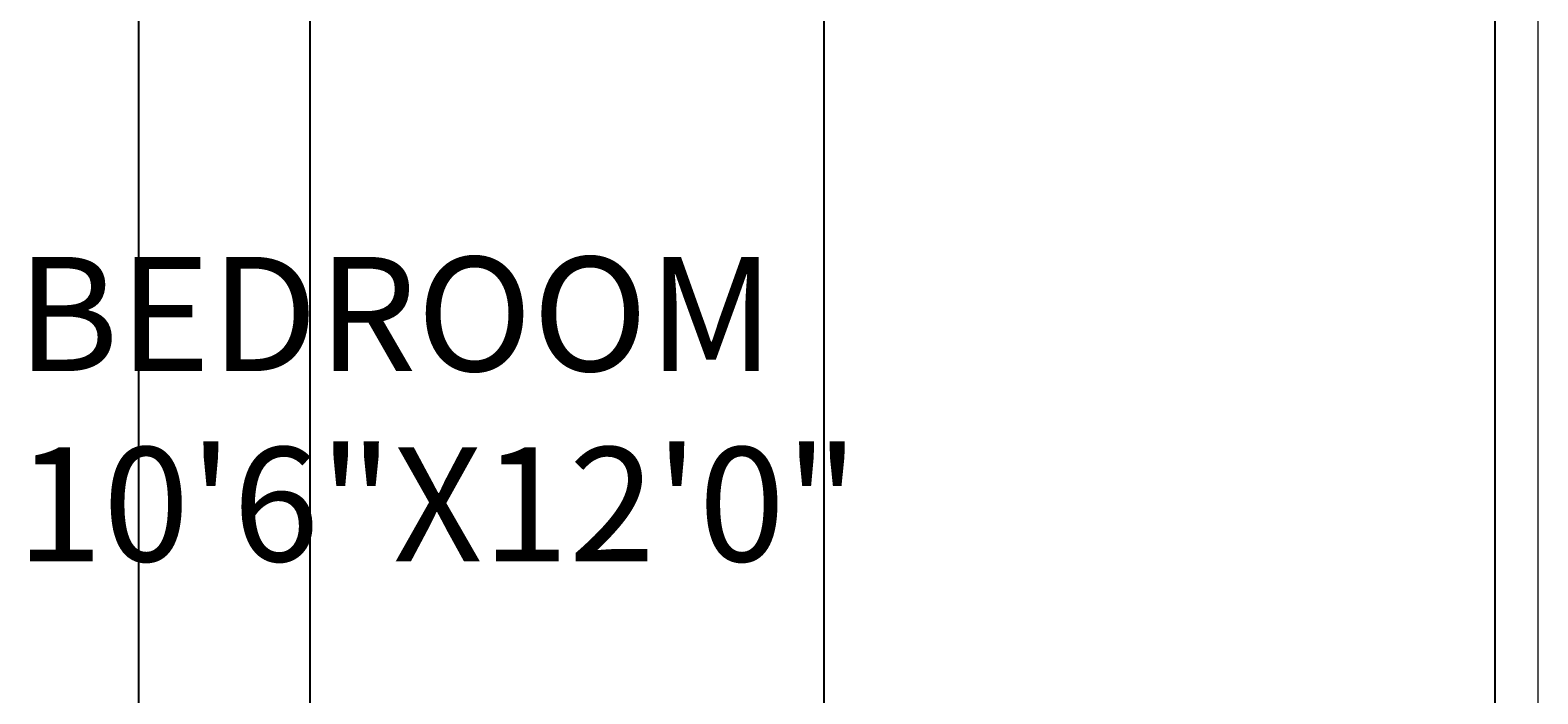
# Model space of a CAD drawing. Units: inches. Extents: x 1088 to 1703, y 668 to 1875.
# Tile 28 of 45: x 1509 to 1588, y 1504 to 1539. Entities that reach past the tile are written whole.
import ezdxf

# ---------------------------------------------------------------- set-up
doc = ezdxf.new("R2010")
doc.units = ezdxf.units.IN
for name, color, linetype, lineweight in [('A-ANNO-DIMS', 2, 'Continuous', 18), ('A-AREA-IDEN', 7, 'Continuous', 18), ('A-DOOR', 4, 'Continuous', 18)]:
    doc.layers.add(name, color=color, linetype=linetype, lineweight=lineweight)
doc.styles.get("Standard").update_dxf_attribs({"font": 'arial.ttf'})
doc.dimstyles.get("Standard").update_dxf_attribs({"dimtxt": 0.18, "dimasz": 0.18, "dimexe": 0.18, "dimexo": 0.0625, "dimgap": 0.09, "dimtad": 0, "dimtih": 1, "dimtoh": 1, "dimdec": 4, "dimzin": 0, "dimdsep": 46, "dimtxsty": 'Standard', "dimcen": 0.09, "dimadec": 0, "dimazin": 0, "dimtfac": 1, "dimtdec": 4, "dimtofl": 0, "dimtmove": 0, "dimatfit": 3, "dimfxl": 1, "dimtolj": 1, "dimtzin": 0, "dimarcsym": 0})

# ---------------------------------------------------------------- blocks, each defined once
blk = doc.blocks.new('*D32')
at = {"layer": 'A-ANNO-DIMS', "color": 0, "lineweight": -2, "transparency": 16777216}
for p, q in [((1550.595, 1373.121), (1550.595, 1857.788)), ((1550.775, 1857.608), (1567.825, 1857.608)), ((1585.665, 1857.608), (1568.614, 1857.608)), ((1585.845, 1360.983), (1585.845, 1857.788))]:
    blk.add_line(p, q, dxfattribs=at)
at = {"layer": 'A-ANNO-DIMS', "color": 0, "transparency": 16777216}
for points in [[(1550.775, 1857.638), (1550.775, 1857.578), (1550.595, 1857.608)], [(1585.665, 1857.638), (1585.665, 1857.578), (1585.845, 1857.608)]]:
    blk.add_solid(points, dxfattribs=at)
at = {"layer": 'Defpoints', "color": 0, "transparency": 16777216}
for p in [(1585.845, 1857.608), (1550.595, 1373.058), (1585.845, 1360.921)]:
    blk.add_point(p, dxfattribs=at)
at = {"layer": 'A-ANNO-DIMS', "color": 0, "transparency": 16777216, "insert": (1568.22, 1857.608), "char_height": 0.18, "attachment_point": 5}
blk.add_mtext('\\A1;35.25', dxfattribs=at)
blk = doc.blocks.new('*D33')
at = {"layer": 'A-ANNO-DIMS', "color": 0, "lineweight": -2, "transparency": 16777216}
for p, q in [((1514.595, 1355.648), (1514.595, 1857.788)), ((1514.775, 1857.608), (1518.946, 1857.608)), ((1523.415, 1857.608), (1519.244, 1857.608)), ((1523.595, 1331.121), (1523.595, 1857.788))]:
    blk.add_line(p, q, dxfattribs=at)
at = {"layer": 'A-ANNO-DIMS', "color": 0, "transparency": 16777216}
for points in [[(1514.775, 1857.638), (1514.775, 1857.578), (1514.595, 1857.608)], [(1523.415, 1857.638), (1523.415, 1857.578), (1523.595, 1857.608)]]:
    blk.add_solid(points, dxfattribs=at)
at = {"layer": 'Defpoints', "color": 0, "transparency": 16777216}
for p in [(1523.595, 1857.608), (1514.595, 1355.585), (1523.595, 1331.058)]:
    blk.add_point(p, dxfattribs=at)
at = {"layer": 'A-ANNO-DIMS', "color": 0, "transparency": 16777216, "insert": (1519.095, 1857.608), "char_height": 0.18, "attachment_point": 5}
blk.add_mtext('\\A1;9', dxfattribs=at)

msp = doc.modelspace()

# ---------------------------------------------------------------- linework, layer by layer
at = {"layer": 'A-DOOR'}
msp.add_line((1588.095, 1539.558), (1588.095, 1478.749), dxfattribs=at)

# ---------------------------------------------------------------- texts
at = {"layer": 'A-AREA-IDEN', "insert": (1508.169, 1526.883), "char_height": 6, "attachment_point": 1}
msp.add_mtext_dynamic_manual_height_columns('BEDROOM\\P10\'6"X12\'0"', width=238.33411, gutter_width=12.5, heights=[0], dxfattribs=at)

# ---------------------------------------------------------------- dimensions: what is measured, and where the dimension line sits
at = {"layer": 'A-ANNO-DIMS'}
for base, p1, p2, override, picture, middle in [((1523.595, 1857.608), (1514.595, 1355.585), (1523.595, 1331.058), {"dimdec": 0, "dimlfac": 1, "dimrnd": 0, "dimzin": 0, "dimdsep": 46, "dimlunit": 2}, '*D33', (1519.095, 1857.608)), ((1585.845, 1857.608), (1550.595, 1373.058), (1585.845, 1360.921), {"dimdec": 2, "dimlfac": 1, "dimrnd": 0, "dimzin": 0, "dimdsep": 46, "dimlunit": 2}, '*D32', (1568.22, 1857.608))]:
    dim = msp.add_linear_dim(base=base, p1=p1, p2=p2, dimstyle='Standard', override=override, dxfattribs=at)
    dim.commit()
    dim.dimension.update_dxf_attribs({"geometry": picture, "text_midpoint": middle})

doc.saveas('drawing.dxf')
